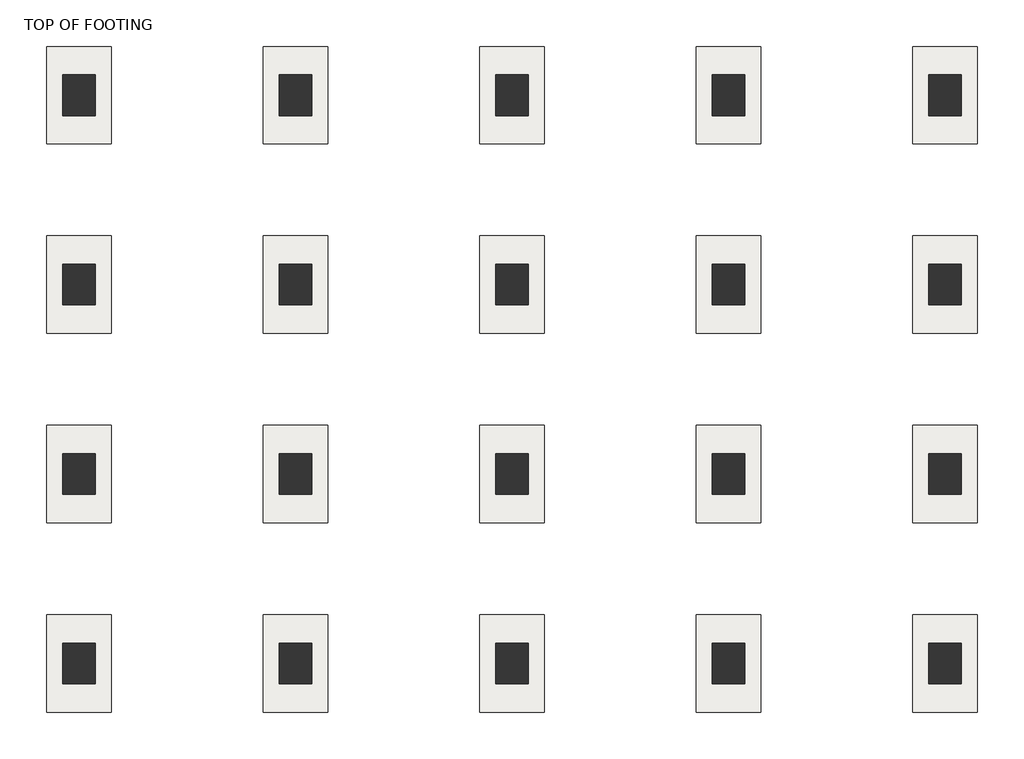
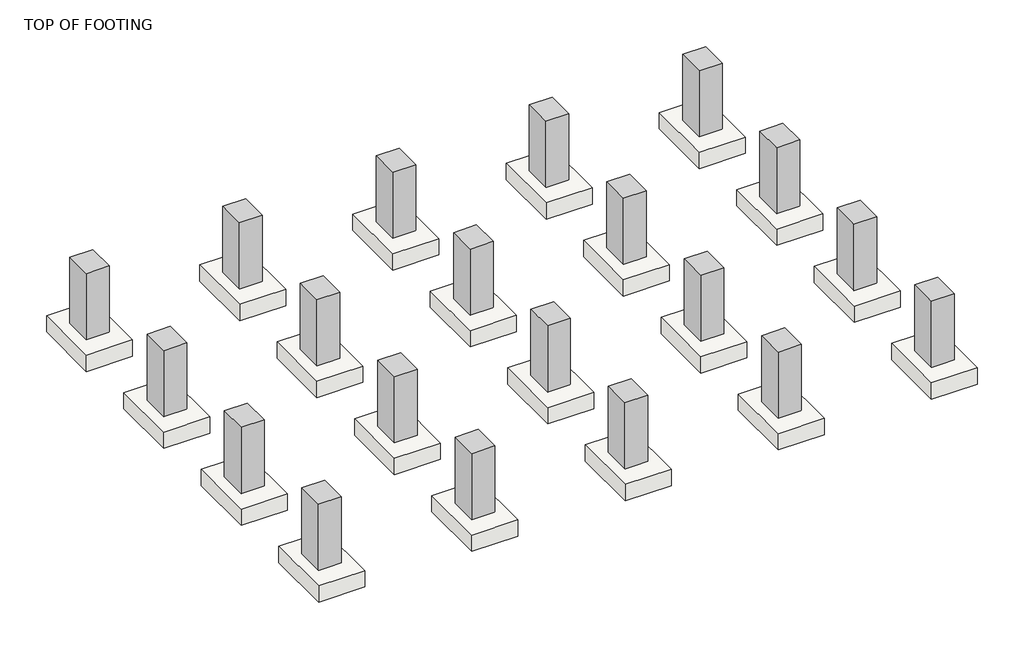
# One storey: 20 columns, 20 slabs.
"""IFC4 building model written with IfcOpenShell, lengths in millimetres."""

from ifc_helpers import new_model, si_unit, frame, origin, place, context, project, spatial, polyline, outline, extrude, transform, mapped, element, save
from components import m_footing_rectangular_1800_x_1200_x_450mm_16ba7ea5

model = new_model("IFC4")

# Units and contexts
model_context = context("Model", 3, world=origin())
ifc_project = project(units=[si_unit("LENGTHUNIT", "METRE", prefix="MILLI")], contexts=[model_context])

# Site, building, storey
site = spatial("IfcSite", under=ifc_project)
building = spatial("IfcBuilding", under=site)
storey = spatial("IfcBuildingStorey", under=building, Name="TOP OF FOOTING", Elevation=-1828.8)

# Columns
placement = place(None, origin())
element("IfcColumn", 1, ObjectType="M_Concrete-Rectangular-Column : 600 x 750mm", at=placement, inside=storey, context=model_context, shape_type="SweptSolid", body=[
    extrude(outline(polyline([(-8630.6620752, 10230.8028699), (-8630.6620752, 9480.8028699), (-9230.6620752, 9480.8028699), (-9230.6620752, 10230.8028699), (-8630.6620752, 10230.8028699)])), frame((0.0, 0.0, -1828.8), z_axis=(0.0, 0.0, 1.0), x_axis=(1.0, 0.0, 0.0)), (0.0, 0.0, 1.0), 1828.8),
])
element("IfcColumn", 2, ObjectType="M_Concrete-Rectangular-Column : 600 x 750mm", at=placement, inside=storey, context=model_context, shape_type="SweptSolid", body=[
    extrude(outline(polyline([(-8630.6620752, 6730.8028699), (-8630.6620752, 5980.8028699), (-9230.6620752, 5980.8028699), (-9230.6620752, 6730.8028699), (-8630.6620752, 6730.8028699)])), frame((0.0, 0.0, -1828.8), z_axis=(0.0, 0.0, 1.0), x_axis=(1.0, 0.0, 0.0)), (0.0, 0.0, 1.0), 1828.8),
])
element("IfcColumn", 3, ObjectType="M_Concrete-Rectangular-Column : 600 x 750mm", at=placement, inside=storey, context=model_context, shape_type="SweptSolid", body=[
    extrude(outline(polyline([(-8630.6620752, 3230.8028699), (-8630.6620752, 2480.8028699), (-9230.6620752, 2480.8028699), (-9230.6620752, 3230.8028699), (-8630.6620752, 3230.8028699)])), frame((0.0, 0.0, -1828.8), z_axis=(0.0, 0.0, 1.0), x_axis=(1.0, 0.0, 0.0)), (0.0, 0.0, 1.0), 1828.8),
])
element("IfcColumn", 4, ObjectType="M_Concrete-Rectangular-Column : 600 x 750mm", at=placement, inside=storey, context=model_context, shape_type="SweptSolid", body=[
    extrude(outline(polyline([(-8630.6620752, -269.1971301), (-8630.6620752, -1019.1971301), (-9230.6620752, -1019.1971301), (-9230.6620752, -269.1971301), (-8630.6620752, -269.1971301)])), frame((0.0, 0.0, -1828.8), z_axis=(0.0, 0.0, 1.0), x_axis=(1.0, 0.0, 0.0)), (0.0, 0.0, 1.0), 1828.8),
])
element("IfcColumn", 5, ObjectType="M_Concrete-Rectangular-Column : 600 x 750mm", at=placement, inside=storey, context=model_context, shape_type="SweptSolid", body=[
    extrude(outline(polyline([(-4630.6620752, 10230.8028699), (-4630.6620752, 9480.8028699), (-5230.6620752, 9480.8028699), (-5230.6620752, 10230.8028699), (-4630.6620752, 10230.8028699)])), frame((0.0, 0.0, -1828.8), z_axis=(0.0, 0.0, 1.0), x_axis=(1.0, 0.0, 0.0)), (0.0, 0.0, 1.0), 1828.8),
])
element("IfcColumn", 6, ObjectType="M_Concrete-Rectangular-Column : 600 x 750mm", at=placement, inside=storey, context=model_context, shape_type="SweptSolid", body=[
    extrude(outline(polyline([(-4630.6620752, 6730.8028699), (-4630.6620752, 5980.8028699), (-5230.6620752, 5980.8028699), (-5230.6620752, 6730.8028699), (-4630.6620752, 6730.8028699)])), frame((0.0, 0.0, -1828.8), z_axis=(0.0, 0.0, 1.0), x_axis=(1.0, 0.0, 0.0)), (0.0, 0.0, 1.0), 1828.8),
])
element("IfcColumn", 7, ObjectType="M_Concrete-Rectangular-Column : 600 x 750mm", at=placement, inside=storey, context=model_context, shape_type="SweptSolid", body=[
    extrude(outline(polyline([(-4630.6620752, 3230.8028699), (-4630.6620752, 2480.8028699), (-5230.6620752, 2480.8028699), (-5230.6620752, 3230.8028699), (-4630.6620752, 3230.8028699)])), frame((0.0, 0.0, -1828.8), z_axis=(0.0, 0.0, 1.0), x_axis=(1.0, 0.0, 0.0)), (0.0, 0.0, 1.0), 1828.8),
])
element("IfcColumn", 8, ObjectType="M_Concrete-Rectangular-Column : 600 x 750mm", at=placement, inside=storey, context=model_context, shape_type="SweptSolid", body=[
    extrude(outline(polyline([(-4630.6620752, -269.1971301), (-4630.6620752, -1019.1971301), (-5230.6620752, -1019.1971301), (-5230.6620752, -269.1971301), (-4630.6620752, -269.1971301)])), frame((0.0, 0.0, -1828.8), z_axis=(0.0, 0.0, 1.0), x_axis=(1.0, 0.0, 0.0)), (0.0, 0.0, 1.0), 1828.8),
])
element("IfcColumn", 9, ObjectType="M_Concrete-Rectangular-Column : 600 x 750mm", at=placement, inside=storey, context=model_context, shape_type="SweptSolid", body=[
    extrude(outline(polyline([(-630.6620752, 10230.8028699), (-630.6620752, 9480.8028699), (-1230.6620752, 9480.8028699), (-1230.6620752, 10230.8028699), (-630.6620752, 10230.8028699)])), frame((0.0, 0.0, -1828.8), z_axis=(0.0, 0.0, 1.0), x_axis=(1.0, 0.0, 0.0)), (0.0, 0.0, 1.0), 1828.8),
])
element("IfcColumn", 10, ObjectType="M_Concrete-Rectangular-Column : 600 x 750mm", at=placement, inside=storey, context=model_context, shape_type="SweptSolid", body=[
    extrude(outline(polyline([(-630.6620752, 6730.8028699), (-630.6620752, 5980.8028699), (-1230.6620752, 5980.8028699), (-1230.6620752, 6730.8028699), (-630.6620752, 6730.8028699)])), frame((0.0, 0.0, -1828.8), z_axis=(0.0, 0.0, 1.0), x_axis=(1.0, 0.0, 0.0)), (0.0, 0.0, 1.0), 1828.8),
])
element("IfcColumn", 11, ObjectType="M_Concrete-Rectangular-Column : 600 x 750mm", at=placement, inside=storey, context=model_context, shape_type="SweptSolid", body=[
    extrude(outline(polyline([(-630.6620752, 3230.8028699), (-630.6620752, 2480.8028699), (-1230.6620752, 2480.8028699), (-1230.6620752, 3230.8028699), (-630.6620752, 3230.8028699)])), frame((0.0, 0.0, -1828.8), z_axis=(0.0, 0.0, 1.0), x_axis=(1.0, 0.0, 0.0)), (0.0, 0.0, 1.0), 1828.8),
])
element("IfcColumn", 12, ObjectType="M_Concrete-Rectangular-Column : 600 x 750mm", at=placement, inside=storey, context=model_context, shape_type="SweptSolid", body=[
    extrude(outline(polyline([(-630.6620752, -269.1971301), (-630.6620752, -1019.1971301), (-1230.6620752, -1019.1971301), (-1230.6620752, -269.1971301), (-630.6620752, -269.1971301)])), frame((0.0, 0.0, -1828.8), z_axis=(0.0, 0.0, 1.0), x_axis=(1.0, 0.0, 0.0)), (0.0, 0.0, 1.0), 1828.8),
])
element("IfcColumn", 13, ObjectType="M_Concrete-Rectangular-Column : 600 x 750mm", at=placement, inside=storey, context=model_context, shape_type="SweptSolid", body=[
    extrude(outline(polyline([(3369.3379248, 10230.8028699), (3369.3379248, 9480.8028699), (2769.3379248, 9480.8028699), (2769.3379248, 10230.8028699), (3369.3379248, 10230.8028699)])), frame((0.0, 0.0, -1828.8), z_axis=(0.0, 0.0, 1.0), x_axis=(1.0, 0.0, 0.0)), (0.0, 0.0, 1.0), 1828.8),
])
element("IfcColumn", 14, ObjectType="M_Concrete-Rectangular-Column : 600 x 750mm", at=placement, inside=storey, context=model_context, shape_type="SweptSolid", body=[
    extrude(outline(polyline([(3369.3379248, 6730.8028699), (3369.3379248, 5980.8028699), (2769.3379248, 5980.8028699), (2769.3379248, 6730.8028699), (3369.3379248, 6730.8028699)])), frame((0.0, 0.0, -1828.8), z_axis=(0.0, 0.0, 1.0), x_axis=(1.0, 0.0, 0.0)), (0.0, 0.0, 1.0), 1828.8),
])
element("IfcColumn", 15, ObjectType="M_Concrete-Rectangular-Column : 600 x 750mm", at=placement, inside=storey, context=model_context, shape_type="SweptSolid", body=[
    extrude(outline(polyline([(3369.3379248, 3230.8028699), (3369.3379248, 2480.8028699), (2769.3379248, 2480.8028699), (2769.3379248, 3230.8028699), (3369.3379248, 3230.8028699)])), frame((0.0, 0.0, -1828.8), z_axis=(0.0, 0.0, 1.0), x_axis=(1.0, 0.0, 0.0)), (0.0, 0.0, 1.0), 1828.8),
])
element("IfcColumn", 16, ObjectType="M_Concrete-Rectangular-Column : 600 x 750mm", at=placement, inside=storey, context=model_context, shape_type="SweptSolid", body=[
    extrude(outline(polyline([(3369.3379248, -269.1971301), (3369.3379248, -1019.1971301), (2769.3379248, -1019.1971301), (2769.3379248, -269.1971301), (3369.3379248, -269.1971301)])), frame((0.0, 0.0, -1828.8), z_axis=(0.0, 0.0, 1.0), x_axis=(1.0, 0.0, 0.0)), (0.0, 0.0, 1.0), 1828.8),
])
element("IfcColumn", 17, ObjectType="M_Concrete-Rectangular-Column : 600 x 750mm", at=placement, inside=storey, context=model_context, shape_type="SweptSolid", body=[
    extrude(outline(polyline([(7369.3379248, 10230.8028699), (7369.3379248, 9480.8028699), (6769.3379248, 9480.8028699), (6769.3379248, 10230.8028699), (7369.3379248, 10230.8028699)])), frame((0.0, 0.0, -1828.8), z_axis=(0.0, 0.0, 1.0), x_axis=(1.0, 0.0, 0.0)), (0.0, 0.0, 1.0), 1828.8),
])
element("IfcColumn", 18, ObjectType="M_Concrete-Rectangular-Column : 600 x 750mm", at=placement, inside=storey, context=model_context, shape_type="SweptSolid", body=[
    extrude(outline(polyline([(7369.3379248, 6730.8028699), (7369.3379248, 5980.8028699), (6769.3379248, 5980.8028699), (6769.3379248, 6730.8028699), (7369.3379248, 6730.8028699)])), frame((0.0, 0.0, -1828.8), z_axis=(0.0, 0.0, 1.0), x_axis=(1.0, 0.0, 0.0)), (0.0, 0.0, 1.0), 1828.8),
])
element("IfcColumn", 19, ObjectType="M_Concrete-Rectangular-Column : 600 x 750mm", at=placement, inside=storey, context=model_context, shape_type="SweptSolid", body=[
    extrude(outline(polyline([(7369.3379248, 3230.8028699), (7369.3379248, 2480.8028699), (6769.3379248, 2480.8028699), (6769.3379248, 3230.8028699), (7369.3379248, 3230.8028699)])), frame((0.0, 0.0, -1828.8), z_axis=(0.0, 0.0, 1.0), x_axis=(1.0, 0.0, 0.0)), (0.0, 0.0, 1.0), 1828.8),
])
element("IfcColumn", 20, ObjectType="M_Concrete-Rectangular-Column : 600 x 750mm", at=placement, inside=storey, context=model_context, shape_type="SweptSolid", body=[
    extrude(outline(polyline([(7369.3379248, -269.1971301), (7369.3379248, -1019.1971301), (6769.3379248, -1019.1971301), (6769.3379248, -269.1971301), (7369.3379248, -269.1971301)])), frame((0.0, 0.0, -1828.8), z_axis=(0.0, 0.0, 1.0), x_axis=(1.0, 0.0, 0.0)), (0.0, 0.0, 1.0), 1828.8),
])

# Slabs
m_footing_rectangular_1800_x_1200_x_450mm_shape = m_footing_rectangular_1800_x_1200_x_450mm_16ba7ea5(model_context)
element("IfcSlab", 21, ObjectType="M_Footing-Rectangular : 1800 x 1200 x 450mm", at=placement, inside=storey, context=model_context, shape_type="MappedRepresentation", body=[
    mapped(m_footing_rectangular_1800_x_1200_x_450mm_shape, transform((-8930.6620752, 9855.8028699, -1828.8), x_axis=(1.0, 0.0, 0.0), y_axis=(0.0, 1.0, 0.0), z_axis=(0.0, 0.0, 1.0))),
])
element("IfcSlab", 22, ObjectType="M_Footing-Rectangular : 1800 x 1200 x 450mm", at=placement, inside=storey, context=model_context, shape_type="MappedRepresentation", body=[
    mapped(m_footing_rectangular_1800_x_1200_x_450mm_shape, transform((-4930.6620752, 9855.8028699, -1828.8), x_axis=(1.0, 0.0, 0.0), y_axis=(0.0, 1.0, 0.0), z_axis=(0.0, 0.0, 1.0))),
])
element("IfcSlab", 23, ObjectType="M_Footing-Rectangular : 1800 x 1200 x 450mm", at=placement, inside=storey, context=model_context, shape_type="MappedRepresentation", body=[
    mapped(m_footing_rectangular_1800_x_1200_x_450mm_shape, transform((-930.6620752, 9855.8028699, -1828.8), x_axis=(1.0, 0.0, 0.0), y_axis=(0.0, 1.0, 0.0), z_axis=(0.0, 0.0, 1.0))),
])
element("IfcSlab", 24, ObjectType="M_Footing-Rectangular : 1800 x 1200 x 450mm", at=placement, inside=storey, context=model_context, shape_type="MappedRepresentation", body=[
    mapped(m_footing_rectangular_1800_x_1200_x_450mm_shape, transform((3069.3379248, 9855.8028699, -1828.8), x_axis=(1.0, 0.0, 0.0), y_axis=(0.0, 1.0, 0.0), z_axis=(0.0, 0.0, 1.0))),
])
element("IfcSlab", 25, ObjectType="M_Footing-Rectangular : 1800 x 1200 x 450mm", at=placement, inside=storey, context=model_context, shape_type="MappedRepresentation", body=[
    mapped(m_footing_rectangular_1800_x_1200_x_450mm_shape, transform((7069.3379248, 9855.8028699, -1828.8), x_axis=(1.0, 0.0, 0.0), y_axis=(0.0, 1.0, 0.0), z_axis=(0.0, 0.0, 1.0))),
])
element("IfcSlab", 26, ObjectType="M_Footing-Rectangular : 1800 x 1200 x 450mm", at=placement, inside=storey, context=model_context, shape_type="MappedRepresentation", body=[
    mapped(m_footing_rectangular_1800_x_1200_x_450mm_shape, transform((7069.3379248, 6355.8028699, -1828.8), x_axis=(1.0, 0.0, 0.0), y_axis=(0.0, 1.0, 0.0), z_axis=(0.0, 0.0, 1.0))),
])
element("IfcSlab", 27, ObjectType="M_Footing-Rectangular : 1800 x 1200 x 450mm", at=placement, inside=storey, context=model_context, shape_type="MappedRepresentation", body=[
    mapped(m_footing_rectangular_1800_x_1200_x_450mm_shape, transform((3069.3379248, 6355.8028699, -1828.8), x_axis=(1.0, 0.0, 0.0), y_axis=(0.0, 1.0, 0.0), z_axis=(0.0, 0.0, 1.0))),
])
element("IfcSlab", 28, ObjectType="M_Footing-Rectangular : 1800 x 1200 x 450mm", at=placement, inside=storey, context=model_context, shape_type="MappedRepresentation", body=[
    mapped(m_footing_rectangular_1800_x_1200_x_450mm_shape, transform((-930.6620752, 6355.8028699, -1828.8), x_axis=(1.0, 0.0, 0.0), y_axis=(0.0, 1.0, 0.0), z_axis=(0.0, 0.0, 1.0))),
])
element("IfcSlab", 29, ObjectType="M_Footing-Rectangular : 1800 x 1200 x 450mm", at=placement, inside=storey, context=model_context, shape_type="MappedRepresentation", body=[
    mapped(m_footing_rectangular_1800_x_1200_x_450mm_shape, transform((-4930.6620752, 6355.8028699, -1828.8), x_axis=(1.0, 0.0, 0.0), y_axis=(0.0, 1.0, 0.0), z_axis=(0.0, 0.0, 1.0))),
])
element("IfcSlab", 30, ObjectType="M_Footing-Rectangular : 1800 x 1200 x 450mm", at=placement, inside=storey, context=model_context, shape_type="MappedRepresentation", body=[
    mapped(m_footing_rectangular_1800_x_1200_x_450mm_shape, transform((-8930.6620752, 6355.8028699, -1828.8), x_axis=(1.0, 0.0, 0.0), y_axis=(0.0, 1.0, 0.0), z_axis=(0.0, 0.0, 1.0))),
])
element("IfcSlab", 31, ObjectType="M_Footing-Rectangular : 1800 x 1200 x 450mm", at=placement, inside=storey, context=model_context, shape_type="MappedRepresentation", body=[
    mapped(m_footing_rectangular_1800_x_1200_x_450mm_shape, transform((-8930.6620752, 2855.8028699, -1828.8), x_axis=(1.0, 0.0, 0.0), y_axis=(0.0, 1.0, 0.0), z_axis=(0.0, 0.0, 1.0))),
])
element("IfcSlab", 32, ObjectType="M_Footing-Rectangular : 1800 x 1200 x 450mm", at=placement, inside=storey, context=model_context, shape_type="MappedRepresentation", body=[
    mapped(m_footing_rectangular_1800_x_1200_x_450mm_shape, transform((-4930.6620752, 2855.8028699, -1828.8), x_axis=(1.0, 0.0, 0.0), y_axis=(0.0, 1.0, 0.0), z_axis=(0.0, 0.0, 1.0))),
])
element("IfcSlab", 33, ObjectType="M_Footing-Rectangular : 1800 x 1200 x 450mm", at=placement, inside=storey, context=model_context, shape_type="MappedRepresentation", body=[
    mapped(m_footing_rectangular_1800_x_1200_x_450mm_shape, transform((-930.6620752, 2855.8028699, -1828.8), x_axis=(1.0, 0.0, 0.0), y_axis=(0.0, 1.0, 0.0), z_axis=(0.0, 0.0, 1.0))),
])
element("IfcSlab", 34, ObjectType="M_Footing-Rectangular : 1800 x 1200 x 450mm", at=placement, inside=storey, context=model_context, shape_type="MappedRepresentation", body=[
    mapped(m_footing_rectangular_1800_x_1200_x_450mm_shape, transform((3069.3379248, 2855.8028699, -1828.8), x_axis=(1.0, 0.0, 0.0), y_axis=(0.0, 1.0, 0.0), z_axis=(0.0, 0.0, 1.0))),
])
element("IfcSlab", 35, ObjectType="M_Footing-Rectangular : 1800 x 1200 x 450mm", at=placement, inside=storey, context=model_context, shape_type="MappedRepresentation", body=[
    mapped(m_footing_rectangular_1800_x_1200_x_450mm_shape, transform((7069.3379248, 2855.8028699, -1828.8), x_axis=(1.0, 0.0, 0.0), y_axis=(0.0, 1.0, 0.0), z_axis=(0.0, 0.0, 1.0))),
])
element("IfcSlab", 36, ObjectType="M_Footing-Rectangular : 1800 x 1200 x 450mm", at=placement, inside=storey, context=model_context, shape_type="MappedRepresentation", body=[
    mapped(m_footing_rectangular_1800_x_1200_x_450mm_shape, transform((7069.3379248, -644.1971301, -1828.8), x_axis=(1.0, 0.0, 0.0), y_axis=(0.0, 1.0, 0.0), z_axis=(0.0, 0.0, 1.0))),
])
element("IfcSlab", 37, ObjectType="M_Footing-Rectangular : 1800 x 1200 x 450mm", at=placement, inside=storey, context=model_context, shape_type="MappedRepresentation", body=[
    mapped(m_footing_rectangular_1800_x_1200_x_450mm_shape, transform((3069.3379248, -644.1971301, -1828.8), x_axis=(1.0, 0.0, 0.0), y_axis=(0.0, 1.0, 0.0), z_axis=(0.0, 0.0, 1.0))),
])
element("IfcSlab", 38, ObjectType="M_Footing-Rectangular : 1800 x 1200 x 450mm", at=placement, inside=storey, context=model_context, shape_type="MappedRepresentation", body=[
    mapped(m_footing_rectangular_1800_x_1200_x_450mm_shape, transform((-930.6620752, -644.1971301, -1828.8), x_axis=(1.0, 0.0, 0.0), y_axis=(0.0, 1.0, 0.0), z_axis=(0.0, 0.0, 1.0))),
])
element("IfcSlab", 39, ObjectType="M_Footing-Rectangular : 1800 x 1200 x 450mm", at=placement, inside=storey, context=model_context, shape_type="MappedRepresentation", body=[
    mapped(m_footing_rectangular_1800_x_1200_x_450mm_shape, transform((-4930.6620752, -644.1971301, -1828.8), x_axis=(1.0, 0.0, 0.0), y_axis=(0.0, 1.0, 0.0), z_axis=(0.0, 0.0, 1.0))),
])
element("IfcSlab", 40, ObjectType="M_Footing-Rectangular : 1800 x 1200 x 450mm", at=placement, inside=storey, context=model_context, shape_type="MappedRepresentation", body=[
    mapped(m_footing_rectangular_1800_x_1200_x_450mm_shape, transform((-8930.6620752, -644.1971301, -1828.8), x_axis=(1.0, 0.0, 0.0), y_axis=(0.0, 1.0, 0.0), z_axis=(0.0, 0.0, 1.0))),
])

save(model, "model.ifc")

# Revit data of these elements
# Grids (mm)
#   "A": line (11430.293, 9855.803) -> (-11716.884, 9855.803)
#   "1": line (-8930.662, 15321.235) -> (-8930.662, -15209.673)
#   "2": line (-4930.662, 15321.235) -> (-4930.662, -15209.673)
#   "3": line (-930.662, 15321.235) -> (-930.662, -15209.673)
#   "4": line (3069.338, 15321.235) -> (3069.338, -15209.673)
#   "5": line (7069.338, 15321.235) -> (7069.338, -15209.673)
#   "B": line (11430.293, 6355.803) -> (-11716.884, 6355.803)
#   "C": line (11430.293, 2855.803) -> (-11716.884, 2855.803)
#   "D": line (11430.293, -644.197) -> (-11716.884, -644.197)
# Type "M_Concrete-Rectangular-Column : 600 x 750mm"
#   b = 1' - 11.62205"
#   h = 2' - 5.52756"
#   Structural Material [instance default] = Concrete, Cast-in-Place gray
# Type "M_Footing-Rectangular : 1800 x 1200 x 450mm"
#   Width = 3' - 11.24409"
#   Length = 5' - 10.86614"
#   Foundation Thickness = 1' - 5.71654"
#   Structural Material [instance default] = Concrete, Cast-in-Place gray
#   Assembly Code = ""
# Elements 1, 2, 3, 4, 5, 6, 7, 8, 9, 10, 11, 12, 13, 14, 15, 16, 17, 18, 19, 20 (IfcColumn, "M_Concrete-Rectangular-Column : 600 x 750mm")
#   Structural Material = Concrete, Cast-in-Place gray
#   Phase Created = New Construction
#   Materials on its faces: "Concrete, Cast-in-Place gray"
# Elements 21, 22, 23, 24, 25, 26, 27, 28, 29, 30, 31, 32, 33, 34, 35, 36, 37, 38, 39, 40 (IfcSlab, "M_Footing-Rectangular : 1800 x 1200 x 450mm")
#   Structural Material = Concrete, Cast-in-Place gray
#   Phase Created = New Construction
#   Materials on its faces: "Concrete, Cast-in-Place gray"
# Materials
#   "Concrete, Cast-in-Place gray": class "Concrete", colour RGB 192 192 192, transparency 0, Description = "Cast-in-place concrete", Cost = 0
